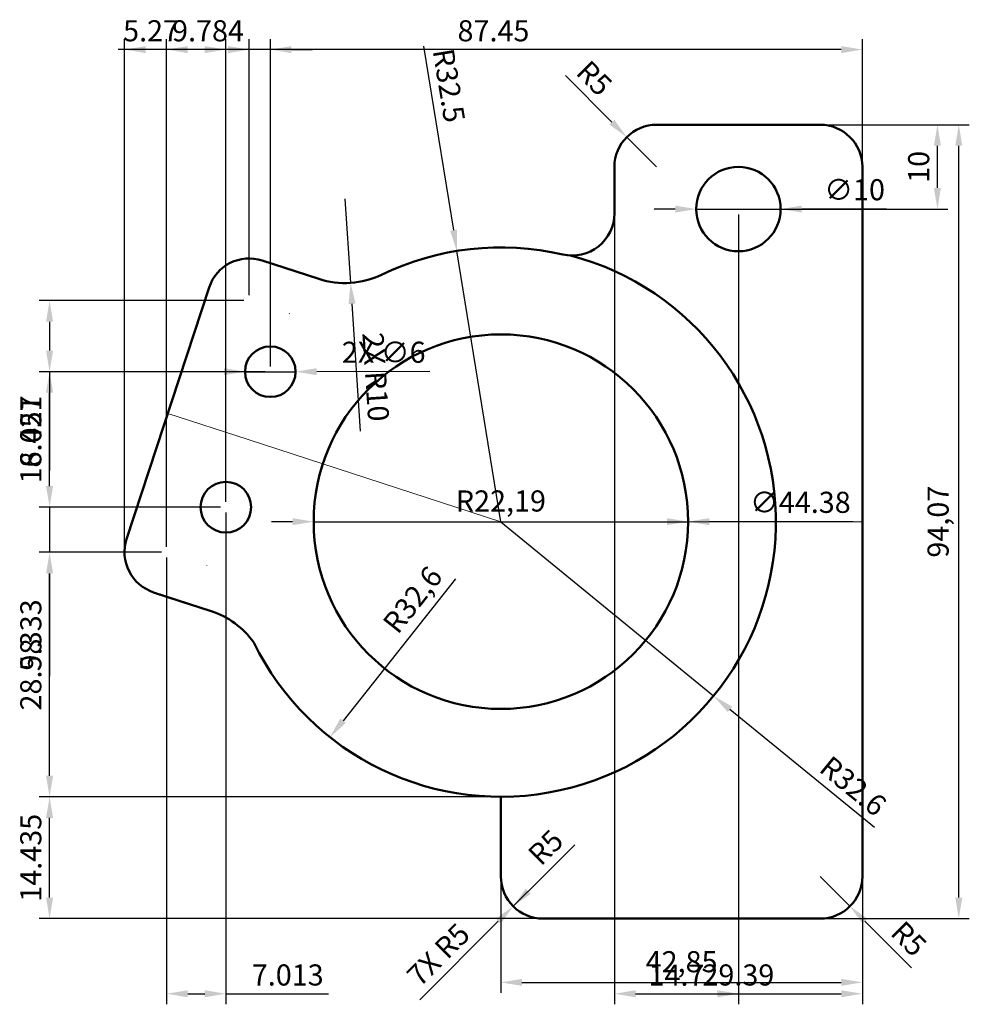
# Model space of a CAD drawing. Units: millimetres. Extents: x 2368 to 2480, y 1613 to 1730.
import ezdxf

# ---------------------------------------------------------------- set-up
doc = ezdxf.new("R2010")
doc.units = ezdxf.units.MM
for name, color, linetype, lineweight in [('M-CONS', 8, 'Continuous', 13), ('M-DIMS', 2, 'Continuous', 25), ('M-OUTL', 7, 'Continuous', 50)]:
    doc.layers.add(name, color=color, linetype=linetype, lineweight=lineweight)
doc.styles.get("Standard").update_dxf_attribs({"font": 'arial.ttf'})
doc.dimstyles.new('ISO-25', dxfattribs={"dimtxt": 2.5, "dimasz": 2.5, "dimexe": 1.25, "dimexo": 0.625, "dimtad": 1, "dimtxsty": 'Standard', "dimcen": 2.5, "dimadec": 0, "dimazin": 0, "dimtfac": 1, "dimtmove": 0, "dimatfit": 3, "dimfxl": 1, "dimarcsym": 0})

# ---------------------------------------------------------------- blocks, each defined once
blk = doc.blocks.new('*D1')
at = {"layer": 'Defpoints', "color": 0, "transparency": 16777216}
for p in [(2467.77, 1670.65), (2424.92, 1633.33), (2467.77, 1616.06)]:
    blk.add_point(p, dxfattribs=at)
at = {"layer": 'M-DIMS', "color": 0, "lineweight": -2, "transparency": 16777216}
for p, q in [((2467.77, 1670.03), (2467.77, 1614.81)), ((2424.92, 1632.71), (2424.92, 1614.81)), ((2427.42, 1616.06), (2465.27, 1616.06))]:
    blk.add_line(p, q, dxfattribs=at)
at = {"layer": 'M-DIMS', "color": 0, "transparency": 16777216}
for points in [[(2427.42, 1616.48), (2427.42, 1615.65), (2424.92, 1616.06)], [(2465.27, 1616.48), (2465.27, 1615.65), (2467.77, 1616.06)]]:
    blk.add_solid(points, dxfattribs=at)
at = {"layer": 'M-DIMS', "color": 0, "transparency": 16777216, "insert": (2446.34, 1618.19), "char_height": 2.5, "attachment_point": 5}
blk.add_mtext('42,85', dxfattribs=at)
blk = doc.blocks.new('*D2')
at = {"layer": 'Defpoints', "color": 0, "transparency": 16777216}
for p in [(2453.07, 1717.69), (2479.2, 1717.69), (2446.34, 1623.62)]:
    blk.add_point(p, dxfattribs=at)
at = {"layer": 'M-DIMS', "color": 0, "lineweight": -2, "transparency": 16777216}
for p, q in [((2453.7, 1717.69), (2480.45, 1717.69)), ((2479.2, 1626.12), (2479.2, 1715.19)), ((2446.97, 1623.62), (2480.45, 1623.62))]:
    blk.add_line(p, q, dxfattribs=at)
at = {"layer": 'M-DIMS', "color": 0, "transparency": 16777216}
for points in [[(2478.78, 1715.19), (2479.62, 1715.19), (2479.2, 1717.69)], [(2478.78, 1626.12), (2479.62, 1626.12), (2479.2, 1623.62)]]:
    blk.add_solid(points, dxfattribs=at)
at = {"layer": 'M-DIMS', "color": 0, "transparency": 16777216, "insert": (2477.07, 1670.65), "char_height": 2.5, "attachment_point": 5, "rotation": 90}
blk.add_mtext('94,07', dxfattribs=at)
blk = doc.blocks.new('*D3')
at = {"layer": 'Defpoints', "color": 0, "transparency": 16777216}
for p in [(2429.92, 1628.62), (2426.38, 1625.08)]:
    blk.add_point(p, dxfattribs=at)
at = {"layer": 'M-DIMS', "color": 0, "lineweight": -2, "transparency": 16777216}
blk.add_line((2433.67, 1632.36), (2428.15, 1626.85), dxfattribs=at)
at = {"layer": 'M-DIMS', "color": 0, "transparency": 16777216}
blk.add_solid([(2427.85, 1627.14), (2428.44, 1626.55), (2426.38, 1625.08)], dxfattribs=at)
at = {"layer": 'M-DIMS', "color": 0, "transparency": 16777216, "insert": (2430.45, 1631.83), "char_height": 2.5, "attachment_point": 5, "rotation": 45}
blk.add_mtext('R5', dxfattribs=at)
blk = doc.blocks.new('*D4')
at = {"layer": 'Defpoints', "color": 0, "transparency": 16777216}
for p in [(2439.84, 1716.22), (2443.38, 1712.69)]:
    blk.add_point(p, dxfattribs=at)
at = {"layer": 'M-DIMS', "color": 0, "lineweight": -2, "transparency": 16777216}
for p, q in [((2432.56, 1723.51), (2438.07, 1717.99)), ((2443.38, 1712.69), (2439.84, 1716.22))]:
    blk.add_line(p, q, dxfattribs=at)
at = {"layer": 'M-DIMS', "color": 0, "transparency": 16777216}
blk.add_solid([(2438.37, 1718.28), (2437.78, 1717.7), (2439.84, 1716.22)], dxfattribs=at)
at = {"layer": 'M-DIMS', "color": 0, "transparency": 16777216, "insert": (2435.77, 1722.97), "char_height": 2.5, "attachment_point": 5, "rotation": 315}
blk.add_mtext('R5', dxfattribs=at)
blk = doc.blocks.new('*D5')
at = {"layer": 'Defpoints', "color": 0, "transparency": 16777216}
for p in [(2462.77, 1628.62), (2466.3, 1625.08)]:
    blk.add_point(p, dxfattribs=at)
at = {"layer": 'M-DIMS', "color": 0, "lineweight": -2, "transparency": 16777216}
for p, q in [((2462.77, 1628.62), (2466.3, 1625.08)), ((2473.59, 1617.8), (2468.07, 1623.31))]:
    blk.add_line(p, q, dxfattribs=at)
at = {"layer": 'M-DIMS', "color": 0, "transparency": 16777216}
blk.add_solid([(2468.37, 1623.61), (2467.78, 1623.02), (2466.3, 1625.08)], dxfattribs=at)
at = {"layer": 'M-DIMS', "color": 0, "transparency": 16777216, "insert": (2473.05, 1621.01), "char_height": 2.5, "attachment_point": 5, "rotation": 315}
blk.add_mtext('R5', dxfattribs=at)
blk = doc.blocks.new('*D6')
at = {"layer": 'Defpoints', "color": 0, "transparency": 16777216}
for p in [(2424.92, 1670.65), (2404.66, 1645.11)]:
    blk.add_point(p, dxfattribs=at)
at = {"layer": 'M-DIMS', "color": 0, "lineweight": -2, "transparency": 16777216}
blk.add_line((2419.53, 1663.86), (2406.21, 1647.07), dxfattribs=at)
at = {"layer": 'M-DIMS', "color": 0, "transparency": 16777216}
blk.add_solid([(2405.88, 1647.33), (2406.54, 1646.81), (2404.66, 1645.11)], dxfattribs=at)
at = {"layer": 'M-DIMS', "color": 0, "transparency": 16777216, "insert": (2414.71, 1661.21), "char_height": 2.5, "attachment_point": 5, "rotation": 51.575}
blk.add_mtext('R32,6', dxfattribs=at)
blk = doc.blocks.new('*D7')
at = {"layer": 'Defpoints', "color": 0, "transparency": 16777216}
for p in [(2424.92, 1670.65), (2447.11, 1670.65)]:
    blk.add_point(p, dxfattribs=at)
at = {"layer": 'M-DIMS', "color": 0, "lineweight": -2, "transparency": 16777216}
blk.add_line((2418.88, 1670.65), (2444.61, 1670.65), dxfattribs=at)
at = {"layer": 'M-DIMS', "color": 0, "transparency": 16777216}
blk.add_solid([(2444.61, 1671.07), (2444.61, 1670.24), (2447.11, 1670.65)], dxfattribs=at)
at = {"layer": 'M-DIMS', "color": 0, "transparency": 16777216, "insert": (2424.92, 1672.78), "char_height": 2.5, "attachment_point": 5}
blk.add_mtext('R22,19', dxfattribs=at)
blk = doc.blocks.new('MOUNT-HOLE-D6')
blk.add_circle((3, 3), 3)
blk = doc.blocks.new('*D9')
at = {"layer": 'Defpoints', "color": 0, "transparency": 16777216}
for p in [(2380.32, 1726.59), (2467.77, 1712.69), (2380.32, 1666.65)]:
    blk.add_point(p, dxfattribs=at)
at = {"layer": 'M-DIMS', "color": 0, "lineweight": -2, "transparency": 16777216}
for p, q in [((2380.32, 1667.28), (2380.32, 1727.84)), ((2467.77, 1713.31), (2467.77, 1727.84)), ((2465.27, 1726.59), (2382.82, 1726.59))]:
    blk.add_line(p, q, dxfattribs=at)
at = {"layer": 'M-DIMS', "color": 0, "transparency": 16777216}
for points in [[(2382.82, 1727), (2382.82, 1726.17), (2380.32, 1726.59)], [(2465.27, 1727), (2465.27, 1726.17), (2467.77, 1726.59)]]:
    blk.add_solid(points, dxfattribs=at)
at = {"layer": 'M-DIMS', "color": 0, "transparency": 16777216, "insert": (2424.04, 1728.49), "char_height": 2.5, "attachment_point": 5}
blk.add_mtext('87.45', dxfattribs=at)
blk = doc.blocks.new('*D10')
at = {"layer": 'Defpoints', "color": 0, "transparency": 16777216}
for p in [(2371.42, 1638.05), (2424.92, 1638.05), (2429.92, 1623.62)]:
    blk.add_point(p, dxfattribs=at)
at = {"layer": 'M-DIMS', "color": 0, "lineweight": -2, "transparency": 16777216}
for p, q in [((2424.29, 1638.05), (2370.17, 1638.05)), ((2371.42, 1626.12), (2371.42, 1635.55)), ((2429.29, 1623.62), (2370.17, 1623.62))]:
    blk.add_line(p, q, dxfattribs=at)
at = {"layer": 'M-DIMS', "color": 0, "transparency": 16777216}
for points in [[(2371, 1635.55), (2371.84, 1635.55), (2371.42, 1638.05)], [(2371, 1626.12), (2371.84, 1626.12), (2371.42, 1623.62)]]:
    blk.add_solid(points, dxfattribs=at)
at = {"layer": 'M-DIMS', "color": 0, "transparency": 16777216, "insert": (2369.52, 1630.83), "char_height": 2.5, "attachment_point": 5, "rotation": 90}
blk.add_mtext('14.435', dxfattribs=at)
blk = doc.blocks.new('*D11')
at = {"layer": 'Defpoints', "color": 0, "transparency": 16777216}
for p in [(2438.38, 1707.19), (2453.08, 1707.69), (2453.08, 1614.72)]:
    blk.add_point(p, dxfattribs=at)
at = {"layer": 'M-DIMS', "color": 0, "lineweight": -2, "transparency": 16777216}
for p, q in [((2453.08, 1707.06), (2453.08, 1613.47)), ((2438.38, 1706.56), (2438.38, 1613.47)), ((2440.88, 1614.72), (2450.58, 1614.72))]:
    blk.add_line(p, q, dxfattribs=at)
at = {"layer": 'M-DIMS', "color": 0, "transparency": 16777216}
for points in [[(2440.88, 1615.13), (2440.88, 1614.3), (2438.38, 1614.72)], [(2450.58, 1615.13), (2450.58, 1614.3), (2453.08, 1614.72)]]:
    blk.add_solid(points, dxfattribs=at)
at = {"layer": 'M-DIMS', "color": 0, "transparency": 16777216, "insert": (2445.73, 1616.6), "char_height": 2.5, "attachment_point": 5}
blk.add_mtext('14.7', dxfattribs=at)
blk = doc.blocks.new('*D12')
at = {"layer": 'Defpoints', "color": 0, "transparency": 16777216}
for p in [(2438.38, 1712.69), (2467.77, 1712.69), (2467.77, 1614.72)]:
    blk.add_point(p, dxfattribs=at)
at = {"layer": 'M-DIMS', "color": 0, "lineweight": -2, "transparency": 16777216}
for p, q in [((2438.38, 1712.06), (2438.38, 1613.47)), ((2467.77, 1712.06), (2467.77, 1613.47)), ((2440.88, 1614.72), (2465.27, 1614.72))]:
    blk.add_line(p, q, dxfattribs=at)
at = {"layer": 'M-DIMS', "color": 0, "transparency": 16777216}
for points in [[(2440.88, 1615.13), (2440.88, 1614.3), (2438.38, 1614.72)], [(2465.27, 1615.13), (2465.27, 1614.3), (2467.77, 1614.72)]]:
    blk.add_solid(points, dxfattribs=at)
at = {"layer": 'M-DIMS', "color": 0, "transparency": 16777216, "insert": (2453.07, 1616.62), "char_height": 2.5, "attachment_point": 5}
blk.add_mtext('29.39', dxfattribs=at)
blk = doc.blocks.new('*D13')
at = {"layer": 'Defpoints', "color": 0, "transparency": 16777216}
for p in [(2462.77, 1717.69), (2476.67, 1717.69), (2453.08, 1707.69)]:
    blk.add_point(p, dxfattribs=at)
at = {"layer": 'M-DIMS', "color": 0, "lineweight": -2, "transparency": 16777216}
for p, q in [((2463.39, 1717.69), (2477.92, 1717.69)), ((2476.67, 1710.19), (2476.67, 1715.19)), ((2453.7, 1707.69), (2477.92, 1707.69))]:
    blk.add_line(p, q, dxfattribs=at)
at = {"layer": 'M-DIMS', "color": 0, "transparency": 16777216}
for points in [[(2476.25, 1715.19), (2477.08, 1715.19), (2476.67, 1717.69)], [(2476.25, 1710.19), (2477.08, 1710.19), (2476.67, 1707.69)]]:
    blk.add_solid(points, dxfattribs=at)
at = {"layer": 'M-DIMS', "color": 0, "transparency": 16777216, "insert": (2474.77, 1712.69), "char_height": 2.5, "attachment_point": 5, "rotation": 90}
blk.add_mtext('10', dxfattribs=at)
blk = doc.blocks.new('*D14')
at = {"layer": 'Defpoints', "color": 0, "transparency": 16777216}
for p in [(2371.42, 1667.03), (2385.3, 1667.03), (2424.92, 1638.05)]:
    blk.add_point(p, dxfattribs=at)
at = {"layer": 'M-DIMS', "color": 0, "lineweight": -2, "transparency": 16777216}
for p, q in [((2384.68, 1667.03), (2370.17, 1667.03)), ((2371.42, 1640.55), (2371.42, 1664.53)), ((2424.29, 1638.05), (2370.17, 1638.05))]:
    blk.add_line(p, q, dxfattribs=at)
at = {"layer": 'M-DIMS', "color": 0, "transparency": 16777216}
for points in [[(2371, 1664.53), (2371.84, 1664.53), (2371.42, 1667.03)], [(2371, 1640.55), (2371.84, 1640.55), (2371.42, 1638.05)]]:
    blk.add_solid(points, dxfattribs=at)
at = {"layer": 'M-DIMS', "color": 0, "transparency": 16777216, "insert": (2369.52, 1652.54), "char_height": 2.5, "attachment_point": 5, "rotation": 90}
blk.add_mtext('28.98', dxfattribs=at)
blk = doc.blocks.new('*D15')
at = {"layer": 'Defpoints', "color": 0, "transparency": 16777216}
for p in [(2392.32, 1672.37), (2385.3, 1667.03), (2392.32, 1614.72)]:
    blk.add_point(p, dxfattribs=at)
at = {"layer": 'M-DIMS', "color": 0, "lineweight": -2, "transparency": 16777216}
for p, q in [((2392.32, 1671.74), (2392.32, 1613.47)), ((2385.3, 1666.41), (2385.3, 1613.47)), ((2387.8, 1614.72), (2389.82, 1614.72)), ((2392.32, 1614.72), (2404.48, 1614.72))]:
    blk.add_line(p, q, dxfattribs=at)
at = {"layer": 'M-DIMS', "color": 0, "transparency": 16777216}
for points in [[(2387.8, 1615.13), (2387.8, 1614.3), (2385.3, 1614.72)], [(2389.82, 1615.13), (2389.82, 1614.3), (2392.32, 1614.72)]]:
    blk.add_solid(points, dxfattribs=at)
at = {"layer": 'M-DIMS', "color": 0, "transparency": 16777216, "insert": (2399.65, 1616.62), "char_height": 2.5, "attachment_point": 5}
blk.add_mtext('7.013', dxfattribs=at)
blk = doc.blocks.new('*D16')
at = {"layer": 'Defpoints', "color": 0, "transparency": 16777216}
for p in [(2392.32, 1672.37), (2371.42, 1667.03), (2385.3, 1667.03)]:
    blk.add_point(p, dxfattribs=at)
at = {"layer": 'M-DIMS', "color": 0, "lineweight": -2, "transparency": 16777216}
for p, q in [((2371.42, 1674.87), (2371.42, 1677.37)), ((2391.69, 1672.37), (2370.17, 1672.37)), ((2371.42, 1672.37), (2371.42, 1667.03)), ((2384.68, 1667.03), (2370.17, 1667.03)), ((2371.42, 1664.53), (2371.42, 1652.35))]:
    blk.add_line(p, q, dxfattribs=at)
at = {"layer": 'M-DIMS', "color": 0, "transparency": 16777216}
for points in [[(2371, 1674.87), (2371.84, 1674.87), (2371.42, 1672.37)], [(2371, 1664.53), (2371.84, 1664.53), (2371.42, 1667.03)]]:
    blk.add_solid(points, dxfattribs=at)
at = {"layer": 'M-DIMS', "color": 0, "transparency": 16777216, "insert": (2369.52, 1657.19), "char_height": 2.5, "attachment_point": 5, "rotation": 90}
blk.add_mtext('5.333', dxfattribs=at)
blk = doc.blocks.new('*D17')
at = {"layer": 'Defpoints', "color": 0, "transparency": 16777216}
for p in [(2392.32, 1726.59), (2397.59, 1688.42), (2392.32, 1672.37)]:
    blk.add_point(p, dxfattribs=at)
at = {"layer": 'M-DIMS', "color": 0, "lineweight": -2, "transparency": 16777216}
for p, q in [((2392.32, 1672.99), (2392.32, 1727.84)), ((2397.59, 1689.05), (2397.59, 1727.84)), ((2389.82, 1726.59), (2379.57, 1726.59)), ((2397.59, 1726.59), (2392.32, 1726.59)), ((2400.09, 1726.59), (2402.59, 1726.59))]:
    blk.add_line(p, q, dxfattribs=at)
at = {"layer": 'M-DIMS', "color": 0, "transparency": 16777216}
for points in [[(2389.82, 1727), (2389.82, 1726.17), (2392.32, 1726.59)], [(2400.09, 1727), (2400.09, 1726.17), (2397.59, 1726.59)]]:
    blk.add_solid(points, dxfattribs=at)
at = {"layer": 'M-DIMS', "color": 0, "transparency": 16777216, "insert": (2383.45, 1728.49), "char_height": 2.5, "attachment_point": 5}
blk.add_mtext('5.27', dxfattribs=at)
blk = doc.blocks.new('*D18')
at = {"layer": 'Defpoints', "color": 0, "transparency": 16777216}
for p in [(2371.42, 1688.42), (2397.59, 1688.42), (2392.32, 1672.37)]:
    blk.add_point(p, dxfattribs=at)
at = {"layer": 'M-DIMS', "color": 0, "lineweight": -2, "transparency": 16777216}
for p, q in [((2396.96, 1688.42), (2370.17, 1688.42)), ((2371.42, 1674.87), (2371.42, 1685.92)), ((2391.69, 1672.37), (2370.17, 1672.37))]:
    blk.add_line(p, q, dxfattribs=at)
at = {"layer": 'M-DIMS', "color": 0, "transparency": 16777216}
for points in [[(2371, 1685.92), (2371.84, 1685.92), (2371.42, 1688.42)], [(2371, 1674.87), (2371.84, 1674.87), (2371.42, 1672.37)]]:
    blk.add_solid(points, dxfattribs=at)
at = {"layer": 'M-DIMS', "color": 0, "transparency": 16777216, "insert": (2369.52, 1680.4), "char_height": 2.5, "attachment_point": 5, "rotation": 90}
blk.add_mtext('16.057', dxfattribs=at)
blk = doc.blocks.new('*D19')
at = {"layer": 'Defpoints', "color": 0, "transparency": 16777216}
for p in [(2385.3, 1726.59), (2395.09, 1696.84), (2385.3, 1667.03)]:
    blk.add_point(p, dxfattribs=at)
at = {"layer": 'M-DIMS', "color": 0, "lineweight": -2, "transparency": 16777216}
for p, q in [((2385.3, 1667.66), (2385.3, 1727.84)), ((2395.09, 1697.47), (2395.09, 1727.84)), ((2392.59, 1726.59), (2387.8, 1726.59))]:
    blk.add_line(p, q, dxfattribs=at)
at = {"layer": 'M-DIMS', "color": 0, "transparency": 16777216}
for points in [[(2387.8, 1727), (2387.8, 1726.17), (2385.3, 1726.59)], [(2392.59, 1727), (2392.59, 1726.17), (2395.09, 1726.59)]]:
    blk.add_solid(points, dxfattribs=at)
at = {"layer": 'M-DIMS', "color": 0, "transparency": 16777216, "insert": (2390.2, 1728.49), "char_height": 2.5, "attachment_point": 5}
blk.add_mtext('9.784', dxfattribs=at)
blk = doc.blocks.new('*D20')
at = {"layer": 'Defpoints', "color": 0, "transparency": 16777216}
for p in [(2395.09, 1696.84), (2371.42, 1688.42), (2397.59, 1688.42)]:
    blk.add_point(p, dxfattribs=at)
at = {"layer": 'M-DIMS', "color": 0, "lineweight": -2, "transparency": 16777216}
for p, q in [((2394.46, 1696.84), (2370.17, 1696.84)), ((2371.42, 1694.34), (2371.42, 1690.92)), ((2396.96, 1688.42), (2370.17, 1688.42)), ((2371.42, 1688.42), (2371.42, 1676.72))]:
    blk.add_line(p, q, dxfattribs=at)
at = {"layer": 'M-DIMS', "color": 0, "transparency": 16777216}
for points in [[(2371, 1694.34), (2371.84, 1694.34), (2371.42, 1696.84)], [(2371, 1690.92), (2371.84, 1690.92), (2371.42, 1688.42)]]:
    blk.add_solid(points, dxfattribs=at)
at = {"layer": 'M-DIMS', "color": 0, "transparency": 16777216, "insert": (2369.52, 1681.32), "char_height": 2.5, "attachment_point": 5, "rotation": 90}
blk.add_mtext('8.421', dxfattribs=at)
blk = doc.blocks.new('*D21')
at = {"layer": 'Defpoints', "color": 0, "transparency": 16777216}
for p in [(2402.73, 1670.65), (2447.11, 1670.65)]:
    blk.add_point(p, dxfattribs=at)
at = {"layer": 'M-DIMS', "color": 0, "lineweight": -2, "transparency": 16777216}
for p, q in [((2400.23, 1670.65), (2397.73, 1670.65)), ((2402.73, 1670.65), (2447.11, 1670.65)), ((2466.63, 1670.65), (2449.61, 1670.65))]:
    blk.add_line(p, q, dxfattribs=at)
at = {"layer": 'M-DIMS', "color": 0, "transparency": 16777216}
for points in [[(2400.23, 1671.07), (2400.23, 1670.24), (2402.73, 1670.65)], [(2449.61, 1671.07), (2449.61, 1670.24), (2447.11, 1670.65)]]:
    blk.add_solid(points, dxfattribs=at)
at = {"layer": 'M-DIMS', "color": 0, "transparency": 16777216, "insert": (2460.42, 1672.62), "char_height": 2.5, "attachment_point": 5, "rotation": 0.0001}
blk.add_mtext('∅44.38', dxfattribs=at)
blk = doc.blocks.new('*D22')
at = {"layer": 'Defpoints', "color": 0, "transparency": 16777216}
for p in [(2424.92, 1670.65), (2450.14, 1650)]:
    blk.add_point(p, dxfattribs=at)
at = {"layer": 'M-DIMS', "color": 0, "lineweight": -2, "transparency": 16777216}
for p, q in [((2424.92, 1670.65), (2450.14, 1650)), ((2469.19, 1634.4), (2452.07, 1648.41))]:
    blk.add_line(p, q, dxfattribs=at)
at = {"layer": 'M-DIMS', "color": 0, "transparency": 16777216}
blk.add_solid([(2452.34, 1648.74), (2451.81, 1648.09), (2450.14, 1650)], dxfattribs=at)
at = {"layer": 'M-DIMS', "color": 0, "transparency": 16777216, "insert": (2466.48, 1639.08), "char_height": 2.5, "attachment_point": 5, "rotation": 320.6885}
blk.add_mtext('R32.6', dxfattribs=at)
blk = doc.blocks.new('*D23')
at = {"layer": 'Defpoints', "color": 0, "transparency": 16777216}
for p in [(2419.7, 1702.73), (2424.92, 1670.65)]:
    blk.add_point(p, dxfattribs=at)
at = {"layer": 'M-DIMS', "color": 0, "lineweight": -2, "transparency": 16777216}
for p, q in [((2415.75, 1726.99), (2419.3, 1705.2)), ((2424.92, 1670.65), (2419.7, 1702.73))]:
    blk.add_line(p, q, dxfattribs=at)
at = {"layer": 'M-DIMS', "color": 0, "transparency": 16777216}
blk.add_solid([(2419.71, 1705.26), (2418.89, 1705.13), (2419.7, 1702.73)], dxfattribs=at)
at = {"layer": 'M-DIMS', "color": 0, "transparency": 16777216, "insert": (2418.45, 1722.28), "char_height": 2.5, "attachment_point": 5, "rotation": 279.238}
blk.add_mtext('R32.5', dxfattribs=at)
blk = doc.blocks.new('*D24')
at = {"layer": 'Defpoints', "color": 0, "transparency": 16777216}
for p in [(2406.43, 1708.92), (2407.11, 1698.95)]:
    blk.add_point(p, dxfattribs=at)
at = {"layer": 'M-DIMS', "color": 0, "lineweight": -2, "transparency": 16777216}
for p, q in [((2406.43, 1708.92), (2407.11, 1698.95)), ((2408.29, 1681.36), (2407.28, 1696.45))]:
    blk.add_line(p, q, dxfattribs=at)
at = {"layer": 'M-DIMS', "color": 0, "transparency": 16777216}
blk.add_solid([(2407.69, 1696.48), (2406.86, 1696.42), (2407.11, 1698.95)], dxfattribs=at)
at = {"layer": 'M-DIMS', "color": 0, "transparency": 16777216, "insert": (2409.77, 1687.78), "char_height": 2.5, "attachment_point": 5, "rotation": 273.8573}
blk.add_mtext('2X R10', dxfattribs=at)
blk = doc.blocks.new('*D25')
at = {"layer": 'Defpoints', "color": 0, "transparency": 16777216}
for p in [(2429.92, 1628.62), (2426.38, 1625.08)]:
    blk.add_point(p, dxfattribs=at)
at = {"layer": 'M-DIMS', "color": 0, "lineweight": -2, "transparency": 16777216}
for p, q in [((2429.92, 1628.62), (2426.38, 1625.08)), ((2415.31, 1614.01), (2424.61, 1623.31))]:
    blk.add_line(p, q, dxfattribs=at)
at = {"layer": 'M-DIMS', "color": 0, "transparency": 16777216}
blk.add_solid([(2424.32, 1623.61), (2424.91, 1623.02), (2426.38, 1625.08)], dxfattribs=at)
at = {"layer": 'M-DIMS', "color": 0, "transparency": 16777216, "insert": (2417.74, 1619.12), "char_height": 2.5, "attachment_point": 5, "rotation": 44.9969}
blk.add_mtext('7X R5', dxfattribs=at)
blk = doc.blocks.new('*D26')
at = {"layer": 'Defpoints', "color": 0, "transparency": 16777216}
for p in [(2448.08, 1707.69), (2458.08, 1707.69)]:
    blk.add_point(p, dxfattribs=at)
at = {"layer": 'M-DIMS', "color": 0, "lineweight": -2, "transparency": 16777216}
for p, q in [((2445.58, 1707.69), (2443.08, 1707.69)), ((2448.08, 1707.69), (2458.08, 1707.69)), ((2470.62, 1707.69), (2460.58, 1707.69))]:
    blk.add_line(p, q, dxfattribs=at)
at = {"layer": 'M-DIMS', "color": 0, "transparency": 16777216}
for points in [[(2445.58, 1708.1), (2445.58, 1707.27), (2448.08, 1707.69)], [(2460.58, 1708.1), (2460.58, 1707.27), (2458.08, 1707.69)]]:
    blk.add_solid(points, dxfattribs=at)
at = {"layer": 'M-DIMS', "color": 0, "transparency": 16777216, "insert": (2466.85, 1709.66), "char_height": 2.5, "attachment_point": 5, "rotation": 0.0006}
blk.add_mtext('∅10', dxfattribs=at)
blk = doc.blocks.new('*D27')
at = {"layer": 'Defpoints', "color": 0, "transparency": 16777216}
for p in [(2394.59, 1688.42), (2400.59, 1688.42)]:
    blk.add_point(p, dxfattribs=at)
at = {"layer": 'M-DIMS', "color": 0, "lineweight": -2, "transparency": 16777216}
for p, q in [((2392.09, 1688.42), (2389.59, 1688.42)), ((2394.59, 1688.42), (2400.59, 1688.42)), ((2416.48, 1688.43), (2403.09, 1688.42))]:
    blk.add_line(p, q, dxfattribs=at)
at = {"layer": 'M-DIMS', "color": 0, "transparency": 16777216}
for points in [[(2392.09, 1688.84), (2392.09, 1688.01), (2394.59, 1688.42)], [(2403.09, 1688.84), (2403.09, 1688.01), (2400.59, 1688.42)]]:
    blk.add_solid(points, dxfattribs=at)
at = {"layer": 'M-DIMS', "color": 0, "transparency": 16777216, "insert": (2411.03, 1690.4), "char_height": 2.5, "attachment_point": 5, "rotation": 0.0079}
blk.add_mtext('2X ∅6', dxfattribs=at)

msp = doc.modelspace()

# ---------------------------------------------------------------- linework, layer by layer
at = {"layer": 'M-CONS'}
for p, q in [((2394.9523, 1680.3951), (2385.4424, 1683.4873)), ((2424.9173, 1670.6519), (2394.9523, 1680.3951)), ((2424.9173, 1670.6519), (2467.7673, 1670.6519))]:
    msp.add_line(p, q, dxfattribs=at)
for centre in [(2395.0888, 1696.8446), (2385.3047, 1667.0337)]:
    msp.add_arc(centre, 5, 341.606159, 342.053537, dxfattribs=at)
at = {"layer": 'M-OUTL'}
for p, q in [((2462.7673, 1717.6869), (2443.3773, 1717.6869)), ((2438.3773, 1712.6869), (2438.3773, 1707.1852)), ((2467.7673, 1712.6869), (2467.7673, 1628.6169)), ((2396.6389, 1701.5983), (2403.3341, 1699.4151)), ((2380.554, 1668.5929), (2390.3381, 1698.4038)), ((2383.7586, 1662.2788), (2388.5004, 1660.737)), ((2383.7586, 1662.2788), (2390.5601, 1660.0672)), ((2424.9173, 1628.6169), (2424.9173, 1638.0519)), ((2462.7673, 1623.6169), (2429.9173, 1623.6169)), ((2462.7673, 1623.6169), (2429.9173, 1623.6169))]:
    msp.add_line(p, q, dxfattribs=at)
for centre, radius in [((2453.0773, 1707.6869), 5), ((2424.9173, 1670.6519), 22.19)]:
    msp.add_circle(centre, radius, dxfattribs=at)
for centre, radius, start, end in [((2443.3773, 1712.6869), 5, 90, 180), ((2462.7673, 1712.6869), 5, 0, 90), ((2433.3773, 1707.1852), 5, 256.961837, 360), ((2424.9173, 1670.6519), 32.6, 206.045602, 75.331301), ((2424.9173, 1670.6519), 32.5, 76.961837, 115.778649), ((2395.0888, 1696.8446), 5, 71.939719, 161.829848), ((2406.4343, 1708.9224), 10, 251.939719, 295.778649), ((2385.3047, 1667.0337), 5, 161.829848, 251.98802), ((2387.468, 1650.5573), 10, 35.312879, 71.98802), ((2429.9173, 1628.6169), 5, 180, 270), ((2462.7673, 1628.6169), 5, 270, 0)]:
    msp.add_arc(centre, radius, start, end, dxfattribs=at)

# ---------------------------------------------------------------- block references
for p in [(2394.587, 1685.424), (2389.317, 1669.367)]:
    msp.add_blockref('MOUNT-HOLE-D6', p, dxfattribs=at)

# ---------------------------------------------------------------- dimensions: what is measured, and where the dimension line sits
at = {"layer": 'M-DIMS'}
for base, p1, p2, override, picture, middle in [((2392.3173, 1726.5869), (2397.5873, 1688.4236), (2392.3173, 1672.3666), {"dimdec": 2, "dimlfac": 1, "dimrnd": 0, "dimzin": 0, "dimdsep": 46, "dimlunit": 2}, '*D17', (2383.4454, 1728.4884)), ((2380.3192, 1726.5869), (2467.7673, 1712.6869), (2380.3192, 1666.6528), {"dimdec": 2, "dimlfac": 1, "dimrnd": 0, "dimzin": 0, "dimdsep": 46, "dimlunit": 2}, '*D9', (2424.0433, 1728.4884)), ((2385.3047, 1726.5869), (2395.0888, 1696.8446), (2385.3047, 1667.0337), {"dimdec": 3, "dimlfac": 1, "dimrnd": 0, "dimzin": 0, "dimdsep": 46, "dimlunit": 2}, '*D19', (2390.1967, 1728.4884)), ((2467.7673, 1614.7169), (2438.3773, 1712.6869), (2467.7673, 1712.6869), {"dimdec": 2, "dimlfac": 1, "dimrnd": 0, "dimzin": 0, "dimdsep": 46, "dimlunit": 2}, '*D12', (2453.0723, 1616.6192)), ((2453.0773, 1614.7169), (2438.3773, 1707.1852), (2453.0773, 1707.6869), {"dimdec": 1, "dimlfac": 1, "dimrnd": 0, "dimzin": 0, "dimdsep": 46, "dimlunit": 2}, '*D11', (2445.7273, 1616.5971)), ((2392.3173, 1614.7169), (2385.3047, 1667.0337), (2392.3173, 1672.3666), {"dimdec": 3, "dimlfac": 1, "dimrnd": 0, "dimzin": 0, "dimdsep": 46, "dimlunit": 2}, '*D15', (2399.6502, 1616.6192)), ((2467.7673, 1616.065), (2424.9173, 1633.3344), (2467.7673, 1670.6519), {"dimclrd": 0, "dimclre": 0, "dimclrt": 0}, '*D1', (2446.3423, 1618.1924))]:
    dim = msp.add_linear_dim(base=base, p1=p1, p2=p2, dimstyle='ISO-25', override=override, dxfattribs=at)
    dim.commit()
    dim.dimension.update_dxf_attribs({"geometry": picture, "text_midpoint": middle})
for center, mpoint, override, picture, middle in [((2424.9173, 1670.6519), (2419.6999, 1702.7304), {"dimdec": 1, "dimlfac": 1, "dimrnd": 0, "dimzin": 0, "dimdsep": 46, "dimlunit": 2}, '*D23', (2416.5695, 1721.9775)), ((2424.9173, 1670.6519), (2447.1073, 1670.6519), {"dimclrd": 0, "dimclre": 0, "dimclrt": 0}, '*D7', (2424.9173, 1670.6519)), ((2424.9173, 1670.6519), (2404.6568, 1645.1124), {"dimclrd": 0, "dimclre": 0, "dimclrt": 0}, '*D6', (2416.3787, 1659.8885)), ((2424.9173, 1670.6519), (2450.1404, 1649.9987), {"dimdec": 1, "dimlfac": 1, "dimrnd": 0, "dimzin": 0, "dimdsep": 46, "dimlunit": 2}, '*D22', (2465.2742, 1637.6067)), ((2429.9173, 1628.6169), (2426.3818, 1625.0814), {"dimclrd": 0, "dimclre": 0, "dimclrt": 0}, '*D3', (2431.7912, 1630.4908))]:
    dim = msp.add_radius_dim(center=center, mpoint=mpoint, dimstyle='ISO-25', override=override, dxfattribs=at)
    dim.commit()
    dim.dimension.update_dxf_attribs({"geometry": picture, "text_midpoint": middle, "dimtype": 164})
for center, mpoint, picture, middle in [((2443.3773, 1712.6869), (2439.8418, 1716.2225), '*D4', (2435.7733, 1722.9728)), ((2462.7673, 1628.6169), (2466.3029, 1625.0814), '*D5', (2473.0532, 1621.0129))]:
    dim = msp.add_radius_dim(center=center, mpoint=mpoint, dimstyle='ISO-25', override={"dimclrd": 0, "dimclre": 0, "dimclrt": 0}, dxfattribs=at)
    dim.commit()
    dim.dimension.update_dxf_attribs({"geometry": picture, "text_midpoint": middle})
for base, p1, p2, override, picture, middle in [((2479.1988, 1717.6869), (2446.3423, 1623.6169), (2453.0723, 1717.6869), {"dimclrd": 0, "dimclre": 0, "dimclrt": 0}, '*D2', (2477.0714, 1670.6519)), ((2476.6673, 1717.6869), (2453.0773, 1707.6869), (2462.7673, 1717.6869), {"dimdec": 0, "dimlfac": 1, "dimrnd": 0, "dimzin": 0, "dimdsep": 46, "dimlunit": 2}, '*D13', (2474.7659, 1712.6869)), ((2371.4192, 1688.4236), (2395.0888, 1696.8446), (2397.5873, 1688.4236), {"dimdec": 3, "dimlfac": 1, "dimrnd": 0, "dimzin": 0, "dimdsep": 46, "dimlunit": 2}, '*D20', (2369.5178, 1681.3201)), ((2371.4192, 1688.4236), (2392.3173, 1672.3666), (2397.5873, 1688.4236), {"dimdec": 3, "dimlfac": 1, "dimrnd": 0, "dimzin": 0, "dimdsep": 46, "dimlunit": 2}, '*D18', (2369.5178, 1680.3951)), ((2371.4192, 1667.0337), (2392.3173, 1672.3666), (2385.3047, 1667.0337), {"dimdec": 3, "dimlfac": 1, "dimrnd": 0, "dimzin": 0, "dimdsep": 46, "dimlunit": 2}, '*D16', (2369.5169, 1657.1906)), ((2371.4192, 1667.0337), (2424.9173, 1638.0519), (2385.3047, 1667.0337), {"dimdec": 2, "dimlfac": 1, "dimrnd": 0, "dimzin": 0, "dimdsep": 46, "dimlunit": 2}, '*D14', (2369.5178, 1652.5428)), ((2371.4192, 1638.0519), (2429.9173, 1623.6169), (2424.9173, 1638.0519), {"dimdec": 3, "dimlfac": 1, "dimrnd": 0, "dimzin": 0, "dimdsep": 46, "dimlunit": 2}, '*D10', (2369.5169, 1630.8344))]:
    dim = msp.add_linear_dim(base=base, p1=p1, p2=p2, angle=90, dimstyle='ISO-25', override=override, dxfattribs=at)
    dim.commit()
    dim.dimension.update_dxf_attribs({"geometry": picture, "text_midpoint": middle})
for p1, p2, override, picture, middle in [((2448.0773, 1707.6869), (2458.0773, 1707.687), {"dimdec": 0, "dimlfac": 1, "dimrnd": 0, "dimzin": 0, "dimdsep": 46, "dimlunit": 2}, '*D26', (2466.8486, 1707.6871)), ((2402.7273, 1670.6519), (2447.1073, 1670.652), {"dimdec": 2, "dimlfac": 1, "dimrnd": 0, "dimzin": 0, "dimdsep": 46, "dimlunit": 2}, '*D21', (2460.4213, 1670.652))]:
    dim = msp.add_diameter_dim_2p(p1=p1, p2=p2, dimstyle='ISO-25', override=override, dxfattribs=at)
    dim.commit()
    dim.dimension.update_dxf_attribs({"geometry": picture, "text_midpoint": middle, "dimtype": 163})
for center, mpoint, text, picture, middle in [((2406.4343, 1708.9224), (2407.107, 1698.945), '2X <>', '*D24', (2409.7653, 1687.7838)), ((2429.9173, 1628.6169), (2426.3816, 1625.0816), '7X <>', '*D25', (2417.739, 1619.1216))]:
    dim = msp.add_radius_dim(center=center, mpoint=mpoint, text=text, dimstyle='ISO-25', override={"dimdec": 0, "dimlfac": 1, "dimrnd": 0, "dimzin": 0, "dimdsep": 46, "dimlunit": 2}, dxfattribs=at)
    dim.commit()
    dim.dimension.update_dxf_attribs({"geometry": picture, "text_midpoint": middle})
dim = msp.add_diameter_dim_2p(p1=(2394.5873, 1688.4232), p2=(2400.5873, 1688.424), text='2X <>', dimstyle='ISO-25', override={"dimdec": 0, "dimlfac": 1, "dimrnd": 0, "dimzin": 0, "dimdsep": 46, "dimlunit": 2}, dxfattribs=at)
dim.commit()
dim.dimension.update_dxf_attribs({"geometry": '*D27', "text_midpoint": (2411.0316, 1688.4254), "dimtype": 163})

doc.saveas('drawing.dxf')
